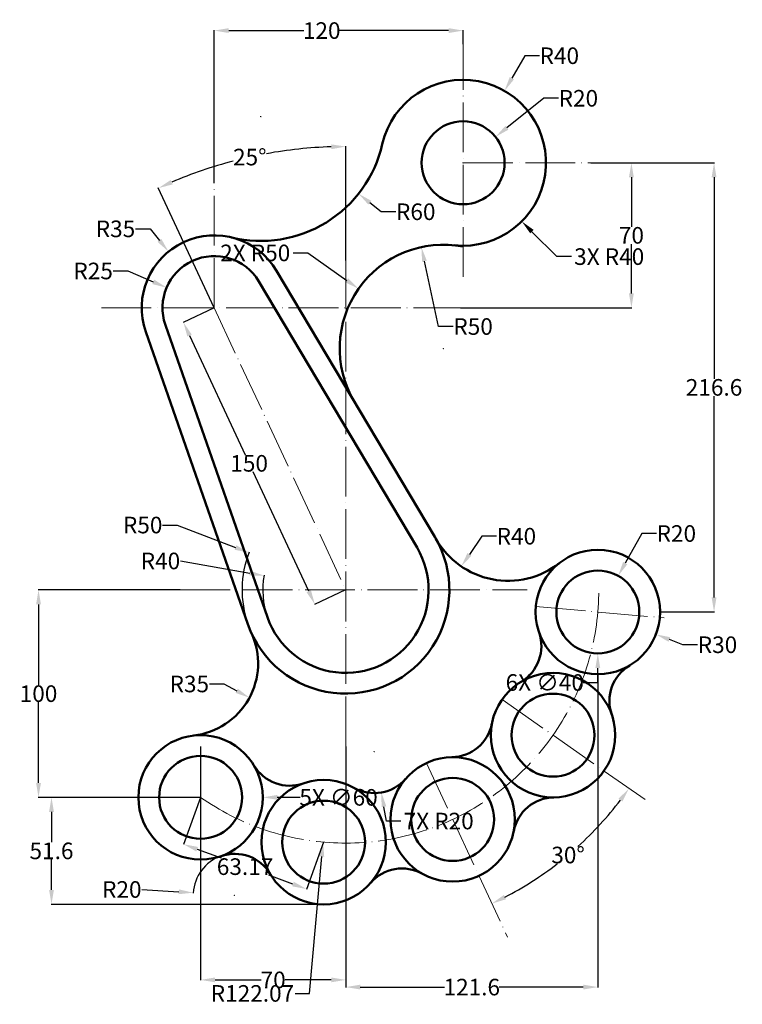
# Model space of a CAD drawing. Units: inches. Extents: x 561 to 910, y 264 to 739.
import ezdxf

# ---------------------------------------------------------------- set-up
doc = ezdxf.new("R2010")
doc.units = ezdxf.units.IN
doc.header["$MEASUREMENT"] = 0
doc.linetypes.add('ACAD_ISO04W100', pattern=[30, 24, -3, 0, -3])
for name, color, linetype, lineweight in [('M-CNTR', 4, 'ACAD_ISO04W100', 18), ('M-DIMS', 2, 'Continuous', 25), ('M-OUTL', 7, 'Continuous', 50)]:
    doc.layers.add(name, color=color, linetype=linetype, lineweight=lineweight)
doc.styles.get("Standard").update_dxf_attribs({"font": 'arial.ttf'})
doc.dimstyles.get("Standard").update_dxf_attribs({"dimtxt": 8, "dimasz": 7, "dimexe": 0.18, "dimexo": 0.0625, "dimgap": 0.09, "dimtad": 0, "dimtih": 1, "dimtoh": 1, "dimdec": 0, "dimzin": 0, "dimdsep": 46, "dimtxsty": 'Standard', "dimcen": 0.09, "dimclrd": 1, "dimclre": 1, "dimadec": 0, "dimazin": 0, "dimtfac": 1, "dimtdec": 0, "dimtofl": 0, "dimtmove": 0, "dimatfit": 3, "dimfxl": 1, "dimtolj": 1, "dimtzin": 0, "dimarcsym": 0})

# ---------------------------------------------------------------- blocks, each defined once
blk = doc.blocks.new('*D1')
at = {"layer": 'Defpoints', "color": 0, "transparency": 16777216}
for p in [(775.26, 733.62), (775.26, 727.02), (655.26, 660.02)]:
    blk.add_point(p, dxfattribs=at)
at = {"layer": 'M-DIMS', "color": 0, "lineweight": -2, "transparency": 16777216}
for p, q in [((655.26, 660.08), (655.26, 733.8)), ((662.26, 733.62), (698.53, 733.62)), ((768.26, 733.62), (715.6, 733.62)), ((775.26, 727.08), (775.26, 733.8))]:
    blk.add_line(p, q, dxfattribs=at)
at = {"layer": 'M-DIMS', "color": 0, "transparency": 16777216}
for points in [[(662.26, 734.79), (662.26, 732.46), (655.26, 733.62)], [(768.26, 734.79), (768.26, 732.46), (775.26, 733.62)]]:
    blk.add_solid(points, dxfattribs=at)
at = {"layer": 'M-DIMS', "color": 0, "transparency": 16777216, "insert": (707.07, 733.62), "char_height": 8, "attachment_point": 5}
blk.add_mtext('\\A1;120', dxfattribs=at)
blk = doc.blocks.new('*D2')
at = {"layer": 'Defpoints', "color": 0, "transparency": 16777216}
for p in [(836.79, 669.91), (856.45, 669.91), (773.89, 599.91)]:
    blk.add_point(p, dxfattribs=at)
at = {"layer": 'M-DIMS', "color": 0, "lineweight": -2, "transparency": 16777216}
for p, q in [((836.85, 669.91), (856.63, 669.91)), ((856.45, 662.91), (856.45, 639.08)), ((856.45, 606.91), (856.45, 630.73)), ((773.95, 599.91), (856.63, 599.91))]:
    blk.add_line(p, q, dxfattribs=at)
at = {"layer": 'M-DIMS', "color": 0, "transparency": 16777216}
for points in [[(855.28, 662.91), (857.61, 662.91), (856.45, 669.91)], [(855.28, 606.91), (857.61, 606.91), (856.45, 599.91)]]:
    blk.add_solid(points, dxfattribs=at)
at = {"layer": 'M-DIMS', "color": 0, "transparency": 16777216, "insert": (856.45, 634.91), "char_height": 8, "attachment_point": 5}
blk.add_mtext('\\A1;70', dxfattribs=at)
blk = doc.blocks.new('*D3')
at = {"layer": 'Defpoints', "color": 0, "transparency": 16777216}
for p in [(677.78, 692.2), (724.83, 654.97)]:
    blk.add_point(p, dxfattribs=at)
at = {"layer": 'M-DIMS', "color": 0, "lineweight": -2, "transparency": 16777216}
for p, q in [((677.69, 692.2), (677.87, 692.2)), ((677.78, 692.11), (677.78, 692.29)), ((735.81, 646.28), (730.32, 650.62)), ((742.81, 646.28), (735.81, 646.28))]:
    blk.add_line(p, q, dxfattribs=at)
at = {"layer": 'M-DIMS', "color": 0, "transparency": 16777216}
blk.add_solid([(731.04, 651.54), (729.59, 649.71), (724.83, 654.97)], dxfattribs=at)
at = {"layer": 'M-DIMS', "color": 0, "transparency": 16777216, "insert": (752.44, 646.28), "char_height": 8, "attachment_point": 5}
blk.add_mtext('\\A1;R60', dxfattribs=at)
blk = doc.blocks.new('*D4')
at = {"layer": 'Defpoints', "color": 0, "transparency": 16777216}
for p in [(755.15, 629.27), (765.75, 580.41)]:
    blk.add_point(p, dxfattribs=at)
at = {"layer": 'M-DIMS', "color": 0, "lineweight": -2, "transparency": 16777216}
for p, q in [((763.47, 590.95), (756.63, 622.43)), ((770.47, 590.95), (763.47, 590.95))]:
    blk.add_line(p, q, dxfattribs=at)
at = {"layer": 'M-DIMS', "color": 0, "transparency": 16777216}
blk.add_solid([(757.77, 622.68), (755.49, 622.19), (755.15, 629.27)], dxfattribs=at)
at = {"layer": 'M-DIMS', "color": 0, "transparency": 16777216, "insert": (780.1, 590.95), "char_height": 8, "attachment_point": 5}
blk.add_mtext('\\A1;R50', dxfattribs=at)
blk = doc.blocks.new('*D5')
at = {"layer": 'Defpoints', "color": 0, "transparency": 16777216}
for p in [(795.26, 704.55), (775.26, 669.91)]:
    blk.add_point(p, dxfattribs=at)
at = {"layer": 'M-DIMS', "color": 0, "lineweight": -2, "transparency": 16777216}
for p, q in [((805.05, 721.5), (798.76, 710.61)), ((812.05, 721.5), (805.05, 721.5)), ((775.17, 669.91), (775.35, 669.91)), ((775.26, 669.82), (775.26, 670))]:
    blk.add_line(p, q, dxfattribs=at)
at = {"layer": 'M-DIMS', "color": 0, "transparency": 16777216}
blk.add_solid([(797.75, 711.2), (799.77, 710.03), (795.26, 704.55)], dxfattribs=at)
at = {"layer": 'M-DIMS', "color": 0, "transparency": 16777216, "insert": (821.68, 721.5), "char_height": 8, "attachment_point": 5}
blk.add_mtext('\\A1;R40', dxfattribs=at)
blk = doc.blocks.new('*D6')
at = {"layer": 'Defpoints', "color": 0, "transparency": 16777216}
for p in [(790.9, 682.38), (775.26, 669.91)]:
    blk.add_point(p, dxfattribs=at)
at = {"layer": 'M-DIMS', "color": 0, "lineweight": -2, "transparency": 16777216}
for p, q in [((814.23, 700.98), (796.37, 686.74)), ((821.23, 700.98), (814.23, 700.98)), ((775.17, 669.91), (775.35, 669.91)), ((775.26, 669.82), (775.26, 670))]:
    blk.add_line(p, q, dxfattribs=at)
at = {"layer": 'M-DIMS', "color": 0, "transparency": 16777216}
blk.add_solid([(795.65, 687.65), (797.1, 685.83), (790.9, 682.38)], dxfattribs=at)
at = {"layer": 'M-DIMS', "color": 0, "transparency": 16777216, "insert": (830.87, 700.98), "char_height": 8, "attachment_point": 5}
blk.add_mtext('\\A1;R20', dxfattribs=at)
blk = doc.blocks.new('*D7')
at = {"layer": 'Defpoints', "color": 0, "transparency": 16777216}
for p in [(687.68, 675.45), (718.66, 622.65), (655.26, 599.91), (718.66, 463.96), (718.66, 388.61)]:
    blk.add_point(p, dxfattribs=at)
at = {"layer": 'M-DIMS', "color": 0, "lineweight": -2, "transparency": 16777216}
for p, q in [((718.66, 622.71), (718.66, 677.89)), ((655.24, 599.96), (628.25, 657.85))]:
    blk.add_line(p, q, dxfattribs=at)
for start, end in [(91.8764, 100.3108), (104.7079, 113.1236)]:
    blk.add_arc((718.66, 463.96), 213.75, start, end, dxfattribs=at)
at = {"layer": 'M-DIMS', "color": 0, "transparency": 16777216}
for points in [[(711.64, 678.76), (711.68, 676.43), (718.66, 677.71)], [(635.19, 659.47), (634.24, 661.6), (628.32, 657.68)]]:
    blk.add_solid(points, dxfattribs=at)
at = {"layer": 'M-DIMS', "color": 0, "transparency": 16777216, "insert": (672.39, 672.64), "char_height": 8, "attachment_point": 5}
blk.add_mtext('\\A1;25°', dxfattribs=at)
blk = doc.blocks.new('*D8')
at = {"layer": 'Defpoints', "color": 0, "transparency": 16777216}
for p in [(633.19, 627.07), (655.26, 599.91)]:
    blk.add_point(p, dxfattribs=at)
at = {"layer": 'M-DIMS', "color": 0, "lineweight": -2, "transparency": 16777216}
for p, q in [((617.29, 638.04), (624.29, 638.04)), ((624.29, 638.04), (628.78, 632.5)), ((655.17, 599.91), (655.35, 599.91)), ((655.26, 599.82), (655.26, 600))]:
    blk.add_line(p, q, dxfattribs=at)
at = {"layer": 'M-DIMS', "color": 0, "transparency": 16777216}
blk.add_solid([(629.69, 633.24), (627.87, 631.77), (633.19, 627.07)], dxfattribs=at)
at = {"layer": 'M-DIMS', "color": 0, "transparency": 16777216, "insert": (607.61, 638.04), "char_height": 8, "attachment_point": 5}
blk.add_mtext('\\A1;R35', dxfattribs=at)
blk = doc.blocks.new('*D9')
at = {"layer": 'Defpoints', "color": 0, "transparency": 16777216}
for p in [(632.27, 609.72), (655.26, 599.91)]:
    blk.add_point(p, dxfattribs=at)
at = {"layer": 'M-DIMS', "color": 0, "lineweight": -2, "transparency": 16777216}
for p, q in [((606.52, 617.73), (613.52, 617.73)), ((613.52, 617.73), (625.83, 612.47)), ((655.17, 599.91), (655.35, 599.91)), ((655.26, 599.82), (655.26, 600))]:
    blk.add_line(p, q, dxfattribs=at)
at = {"layer": 'M-DIMS', "color": 0, "transparency": 16777216}
blk.add_solid([(626.29, 613.54), (625.38, 611.4), (632.27, 609.72)], dxfattribs=at)
at = {"layer": 'M-DIMS', "color": 0, "transparency": 16777216, "insert": (596.84, 617.73), "char_height": 8, "attachment_point": 5}
blk.add_mtext('\\A1;R25', dxfattribs=at)
blk = doc.blocks.new('*D10')
at = {"layer": 'Defpoints', "color": 0, "transparency": 16777216}
for p in [(655.26, 599.91), (718.66, 463.96), (703.77, 457.02)]:
    blk.add_point(p, dxfattribs=at)
at = {"layer": 'M-DIMS', "color": 0, "lineweight": -2, "transparency": 16777216}
for p, q in [((655.21, 599.88), (640.21, 592.89)), ((643.33, 586.62), (670.12, 529.17)), ((700.81, 463.36), (674.02, 520.82)), ((718.6, 463.93), (703.6, 456.94))]:
    blk.add_line(p, q, dxfattribs=at)
at = {"layer": 'M-DIMS', "color": 0, "transparency": 16777216}
for points in [[(644.39, 587.11), (642.27, 586.13), (640.37, 592.96)], [(701.87, 463.85), (699.75, 462.87), (703.77, 457.02)]]:
    blk.add_solid(points, dxfattribs=at)
at = {"layer": 'M-DIMS', "color": 0, "transparency": 16777216, "insert": (672.07, 524.99), "char_height": 8, "attachment_point": 5}
blk.add_mtext('\\A1;150', dxfattribs=at)
blk = doc.blocks.new('*D11')
at = {"layer": 'Defpoints', "color": 0, "transparency": 16777216}
for p in [(671.99, 481.92), (718.66, 463.96)]:
    blk.add_point(p, dxfattribs=at)
at = {"layer": 'M-DIMS', "color": 0, "lineweight": -2, "transparency": 16777216}
for p, q in [((630.36, 495.25), (637.36, 495.25)), ((637.36, 495.25), (665.46, 484.43)), ((718.57, 463.96), (718.75, 463.96)), ((718.66, 463.87), (718.66, 464.05))]:
    blk.add_line(p, q, dxfattribs=at)
blk.add_arc((718.66, 463.96), 50, 158.745, 199.1892, dxfattribs=at)
at = {"layer": 'M-DIMS', "color": 0, "transparency": 16777216}
blk.add_solid([(665.88, 485.52), (665.04, 483.34), (671.99, 481.92)], dxfattribs=at)
at = {"layer": 'M-DIMS', "color": 0, "transparency": 16777216, "insert": (620.73, 495.25), "char_height": 8, "attachment_point": 5}
blk.add_mtext('\\A1;R50', dxfattribs=at)
blk = doc.blocks.new('*D12')
at = {"layer": 'Defpoints', "color": 0, "transparency": 16777216}
for p in [(679.26, 470.87), (718.66, 463.96)]:
    blk.add_point(p, dxfattribs=at)
at = {"layer": 'M-DIMS', "color": 0, "lineweight": -2, "transparency": 16777216}
for p, q in [((638.94, 477.93), (672.36, 472.07)), ((718.57, 463.96), (718.75, 463.96)), ((718.66, 463.87), (718.66, 464.05))]:
    blk.add_line(p, q, dxfattribs=at)
blk.add_arc((718.66, 463.96), 40, 169.8016, 199.1713, dxfattribs=at)
at = {"layer": 'M-DIMS', "color": 0, "transparency": 16777216}
blk.add_solid([(672.56, 473.22), (672.16, 470.93), (679.26, 470.87)], dxfattribs=at)
at = {"layer": 'M-DIMS', "color": 0, "transparency": 16777216, "insert": (629.3, 477.93), "char_height": 8, "attachment_point": 5}
blk.add_mtext('\\A1;R40', dxfattribs=at)
blk = doc.blocks.new('*D13')
at = {"layer": 'Defpoints', "color": 0, "transparency": 16777216}
for p in [(796.96, 508.33), (774.38, 475.31)]:
    blk.add_point(p, dxfattribs=at)
at = {"layer": 'M-DIMS', "color": 0, "lineweight": -2, "transparency": 16777216}
for p, q in [((784.34, 489.86), (778.33, 481.09)), ((791.34, 489.86), (784.34, 489.86))]:
    blk.add_line(p, q, dxfattribs=at)
at = {"layer": 'M-DIMS', "color": 0, "transparency": 16777216}
blk.add_solid([(777.37, 481.75), (779.3, 480.43), (774.38, 475.31)], dxfattribs=at)
at = {"layer": 'M-DIMS', "color": 0, "transparency": 16777216, "insert": (800.97, 489.86), "char_height": 8, "attachment_point": 5}
blk.add_mtext('\\A1;R40', dxfattribs=at)
blk = doc.blocks.new('*D14')
at = {"layer": 'Defpoints', "color": 0, "transparency": 16777216}
for p in [(641.38, 428.55), (672.23, 412.02)]:
    blk.add_point(p, dxfattribs=at)
at = {"layer": 'M-DIMS', "color": 0, "lineweight": -2, "transparency": 16777216}
for p, q in [((652.89, 418.63), (659.89, 418.63)), ((659.89, 418.63), (666.06, 415.33))]:
    blk.add_line(p, q, dxfattribs=at)
at = {"layer": 'M-DIMS', "color": 0, "transparency": 16777216}
blk.add_solid([(666.61, 416.36), (665.51, 414.3), (672.23, 412.02)], dxfattribs=at)
at = {"layer": 'M-DIMS', "color": 0, "transparency": 16777216, "insert": (643.22, 418.63), "char_height": 8, "attachment_point": 5}
blk.add_mtext('\\A1;R35', dxfattribs=at)
blk = doc.blocks.new('*D15')
at = {"layer": 'Defpoints', "color": 0, "transparency": 16777216}
for p in [(638.93, 463.96), (570.49, 363.96), (648.66, 363.96)]:
    blk.add_point(p, dxfattribs=at)
at = {"layer": 'M-DIMS', "color": 0, "lineweight": -2, "transparency": 16777216}
for p, q in [((638.87, 463.96), (570.31, 463.96)), ((570.49, 456.96), (570.49, 418.14)), ((570.49, 370.96), (570.49, 409.79)), ((648.59, 363.96), (570.31, 363.96))]:
    blk.add_line(p, q, dxfattribs=at)
at = {"layer": 'M-DIMS', "color": 0, "transparency": 16777216}
for points in [[(569.32, 456.96), (571.66, 456.96), (570.49, 463.96)], [(569.32, 370.96), (571.66, 370.96), (570.49, 363.96)]]:
    blk.add_solid(points, dxfattribs=at)
at = {"layer": 'M-DIMS', "color": 0, "transparency": 16777216, "insert": (570.49, 413.96), "char_height": 8, "attachment_point": 5}
blk.add_mtext('\\A1;100', dxfattribs=at)
blk = doc.blocks.new('*D16')
at = {"layer": 'Defpoints', "color": 0, "transparency": 16777216}
for p in [(850.04, 470.76), (840.26, 453.32)]:
    blk.add_point(p, dxfattribs=at)
at = {"layer": 'M-DIMS', "color": 0, "lineweight": -2, "transparency": 16777216}
for p, q in [((861.49, 491.16), (853.47, 476.87)), ((868.49, 491.16), (861.49, 491.16)), ((840.17, 453.32), (840.35, 453.32)), ((840.26, 453.23), (840.26, 453.41))]:
    blk.add_line(p, q, dxfattribs=at)
at = {"layer": 'M-DIMS', "color": 0, "transparency": 16777216}
blk.add_solid([(852.45, 477.44), (854.49, 476.3), (850.04, 470.76)], dxfattribs=at)
at = {"layer": 'M-DIMS', "color": 0, "transparency": 16777216, "insert": (878.12, 491.16), "char_height": 8, "attachment_point": 5}
blk.add_mtext('\\A1;R20', dxfattribs=at)
blk = doc.blocks.new('*D17')
at = {"layer": 'Defpoints', "color": 0, "transparency": 16777216}
for p in [(840.26, 453.32), (868.26, 442.56)]:
    blk.add_point(p, dxfattribs=at)
at = {"layer": 'M-DIMS', "color": 0, "lineweight": -2, "transparency": 16777216}
for p, q in [((840.17, 453.32), (840.35, 453.32)), ((840.26, 453.23), (840.26, 453.41)), ((881.33, 437.54), (874.8, 440.05)), ((888.33, 437.54), (881.33, 437.54))]:
    blk.add_line(p, q, dxfattribs=at)
at = {"layer": 'M-DIMS', "color": 0, "transparency": 16777216}
blk.add_solid([(875.21, 441.14), (874.38, 438.96), (868.26, 442.56)], dxfattribs=at)
at = {"layer": 'M-DIMS', "color": 0, "transparency": 16777216, "insert": (897.97, 437.54), "char_height": 8, "attachment_point": 5}
blk.add_mtext('\\A1;R30', dxfattribs=at)
blk = doc.blocks.new('*D18')
at = {"layer": 'Defpoints', "color": 0, "transparency": 16777216}
for p in [(794.07, 411.15), (757.57, 380.52), (864.91, 361.55), (814.35, 327.3), (796.73, 296.54)]:
    blk.add_point(p, dxfattribs=at)
at = {"layer": 'M-DIMS', "color": 0, "lineweight": -2, "transparency": 16777216}
for start, end in [(312.1829, 322.5957), (297.4043, 307.7131)]:
    blk.add_arc((718.66, 463.96), 166.83, start, end, dxfattribs=at)
at = {"layer": 'M-DIMS', "color": 0, "transparency": 16777216}
for points in [[(850.24, 363.31), (852.12, 361.94), (855.31, 368.27)], [(795.96, 314.81), (794.93, 316.9), (789.16, 312.76)]]:
    blk.add_solid(points, dxfattribs=at)
at = {"layer": 'M-DIMS', "color": 0, "transparency": 16777216, "insert": (825.89, 336.16), "char_height": 8, "attachment_point": 5}
blk.add_mtext('\\A1;30°', dxfattribs=at)
blk = doc.blocks.new('*D19')
at = {"layer": 'Defpoints', "color": 0, "transparency": 16777216}
for p in [(648.66, 388.61), (718.66, 388.61), (648.66, 275.95)]:
    blk.add_point(p, dxfattribs=at)
at = {"layer": 'M-DIMS', "color": 0, "lineweight": -2, "transparency": 16777216}
for p, q in [((648.66, 388.55), (648.66, 275.77)), ((718.66, 388.55), (718.66, 275.77)), ((655.66, 275.95), (677.88, 275.95)), ((711.66, 275.95), (689.43, 275.95))]:
    blk.add_line(p, q, dxfattribs=at)
at = {"layer": 'M-DIMS', "color": 0, "transparency": 16777216}
for points in [[(655.66, 277.12), (655.66, 274.79), (648.66, 275.95)], [(711.66, 277.12), (711.66, 274.79), (718.66, 275.95)]]:
    blk.add_solid(points, dxfattribs=at)
at = {"layer": 'M-DIMS', "color": 0, "transparency": 16777216, "insert": (683.66, 275.95), "char_height": 8, "attachment_point": 5}
blk.add_mtext('\\A1;70', dxfattribs=at)
blk = doc.blocks.new('*D20')
at = {"layer": 'Defpoints', "color": 0, "transparency": 16777216}
for p in [(645.12, 317.99), (665.08, 316.74)]:
    blk.add_point(p, dxfattribs=at)
at = {"layer": 'M-DIMS', "color": 0, "lineweight": -2, "transparency": 16777216}
for p, q in [((620.29, 319.55), (638.14, 318.43)), ((664.99, 316.74), (665.17, 316.74)), ((665.08, 316.65), (665.08, 316.83))]:
    blk.add_line(p, q, dxfattribs=at)
blk.add_arc((665.08, 316.74), 20, 109.3582, 176.9159, dxfattribs=at)
at = {"layer": 'M-DIMS', "color": 0, "transparency": 16777216}
blk.add_solid([(638.21, 319.6), (638.06, 317.27), (645.12, 317.99)], dxfattribs=at)
at = {"layer": 'M-DIMS', "color": 0, "transparency": 16777216, "insert": (610.66, 319.55), "char_height": 8, "attachment_point": 5}
blk.add_mtext('\\A1;R20', dxfattribs=at)
blk = doc.blocks.new('MOUNT-NODE-OD60-ID40')
for radius in [30, 20]:
    blk.add_circle((30, 30), radius)
blk = doc.blocks.new('*D22')
at = {"layer": 'Defpoints', "color": 0, "transparency": 16777216}
for p in [(840.26, 423.32), (718.66, 388.61), (840.26, 272.49)]:
    blk.add_point(p, dxfattribs=at)
at = {"layer": 'M-DIMS', "color": 1, "lineweight": -2, "transparency": 16777216}
for p, q in [((840.26, 423.26), (840.26, 272.31)), ((718.66, 388.55), (718.66, 272.31)), ((725.66, 272.49), (766.25, 272.49)), ((833.26, 272.49), (792.67, 272.49))]:
    blk.add_line(p, q, dxfattribs=at)
at = {"layer": 'M-DIMS', "color": 1, "transparency": 16777216}
for points in [[(725.66, 273.66), (725.66, 271.33), (718.66, 272.49)], [(833.26, 273.66), (833.26, 271.33), (840.26, 272.49)]]:
    blk.add_solid(points, dxfattribs=at)
at = {"layer": 'M-DIMS', "color": 0, "transparency": 16777216, "insert": (779.46, 272.49), "char_height": 8, "attachment_point": 5}
blk.add_mtext('\\A1;121.6', dxfattribs=at)
blk = doc.blocks.new('*D23')
at = {"layer": 'Defpoints', "color": 0, "transparency": 16777216}
for p in [(618.66, 363.96), (576.75, 312.36), (708.02, 312.36)]:
    blk.add_point(p, dxfattribs=at)
at = {"layer": 'M-DIMS', "color": 1, "lineweight": -2, "transparency": 16777216}
for p, q in [((618.59, 363.96), (576.57, 363.96)), ((576.75, 356.96), (576.75, 342.34)), ((576.75, 319.36), (576.75, 333.99)), ((707.96, 312.36), (576.57, 312.36))]:
    blk.add_line(p, q, dxfattribs=at)
at = {"layer": 'M-DIMS', "color": 1, "transparency": 16777216}
for points in [[(575.58, 356.96), (577.91, 356.96), (576.75, 363.96)], [(575.58, 319.36), (577.91, 319.36), (576.75, 312.36)]]:
    blk.add_solid(points, dxfattribs=at)
at = {"layer": 'M-DIMS', "color": 0, "transparency": 16777216, "insert": (576.75, 338.16), "char_height": 8, "attachment_point": 5}
blk.add_mtext('\\A1;51.6', dxfattribs=at)
blk = doc.blocks.new('*D24')
at = {"layer": 'Defpoints', "color": 0, "transparency": 16777216}
for p in [(836.79, 669.91), (870.26, 453.32), (896.31, 453.32)]:
    blk.add_point(p, dxfattribs=at)
at = {"layer": 'M-DIMS', "color": 1, "lineweight": -2, "transparency": 16777216}
for p, q in [((836.85, 669.91), (896.49, 669.91)), ((896.31, 662.91), (896.31, 565.79)), ((896.31, 460.32), (896.31, 557.44)), ((870.32, 453.32), (896.49, 453.32))]:
    blk.add_line(p, q, dxfattribs=at)
at = {"layer": 'M-DIMS', "color": 1, "transparency": 16777216}
for points in [[(895.14, 662.91), (897.48, 662.91), (896.31, 669.91)], [(895.14, 460.32), (897.48, 460.32), (896.31, 453.32)]]:
    blk.add_solid(points, dxfattribs=at)
at = {"layer": 'M-DIMS', "color": 0, "transparency": 16777216, "insert": (896.31, 561.61), "char_height": 8, "attachment_point": 5}
blk.add_mtext('\\A1;216.6', dxfattribs=at)
blk = doc.blocks.new('*D25')
at = {"layer": 'Defpoints', "color": 0, "transparency": 16777216}
for p in [(648.66, 363.96), (708.02, 342.36), (640.43, 341.36)]:
    blk.add_point(p, dxfattribs=at)
at = {"layer": 'M-DIMS', "color": 1, "lineweight": -2, "transparency": 16777216}
for p, q in [((648.64, 363.9), (640.37, 341.19)), ((708, 342.3), (699.73, 319.59)), ((647.01, 338.97), (658.63, 334.74)), ((693.22, 322.15), (681.59, 326.38))]:
    blk.add_line(p, q, dxfattribs=at)
at = {"layer": 'M-DIMS', "color": 1, "transparency": 16777216}
for points in [[(647.41, 340.06), (646.61, 337.87), (640.43, 341.36)], [(693.62, 323.25), (692.82, 321.06), (699.79, 319.76)]]:
    blk.add_solid(points, dxfattribs=at)
at = {"layer": 'M-DIMS', "color": 0, "transparency": 16777216, "insert": (670.11, 330.56), "char_height": 8, "attachment_point": 5}
blk.add_mtext('\\A1;63.17', dxfattribs=at)
blk = doc.blocks.new('*D26')
at = {"layer": 'Defpoints', "color": 0, "transparency": 16777216}
for p in [(718.66, 463.96), (707.75, 342.38)]:
    blk.add_point(p, dxfattribs=at)
at = {"layer": 'M-DIMS', "color": 1, "lineweight": -2, "transparency": 16777216}
for p, q in [((718.57, 463.96), (718.75, 463.96)), ((718.66, 463.87), (718.66, 464.05)), ((701.21, 269.44), (707.12, 335.41)), ((694.21, 269.44), (701.21, 269.44))]:
    blk.add_line(p, q, dxfattribs=at)
at = {"layer": 'M-DIMS', "color": 1, "transparency": 16777216}
blk.add_solid([(705.96, 335.52), (708.29, 335.31), (707.75, 342.38)], dxfattribs=at)
at = {"layer": 'M-DIMS', "color": 0, "transparency": 16777216, "insert": (673.68, 269.44), "char_height": 8, "attachment_point": 5}
blk.add_mtext('\\A1;R122.07', dxfattribs=at)
blk = doc.blocks.new('*D27')
at = {"layer": 'Defpoints', "color": 0, "transparency": 16777216}
for p in [(724.85, 609.17), (765.75, 580.41)]:
    blk.add_point(p, dxfattribs=at)
at = {"layer": 'M-DIMS', "color": 1, "lineweight": -2, "transparency": 16777216}
for p, q in [((693.31, 626.43), (700.31, 626.43)), ((700.31, 626.43), (719.13, 613.2)), ((765.66, 580.41), (765.84, 580.41)), ((765.75, 580.32), (765.75, 580.5))]:
    blk.add_line(p, q, dxfattribs=at)
at = {"layer": 'M-DIMS', "color": 1, "transparency": 16777216}
blk.add_solid([(719.8, 614.15), (718.45, 612.24), (724.85, 609.17)], dxfattribs=at)
at = {"layer": 'M-DIMS', "color": 0, "transparency": 16777216, "insert": (675.01, 626.43), "char_height": 8, "attachment_point": 5}
blk.add_mtext('\\A1;2X R50', dxfattribs=at)
blk = doc.blocks.new('*D28')
at = {"layer": 'Defpoints', "color": 0, "transparency": 16777216}
for p in [(775.26, 669.91), (803.55, 641.62)]:
    blk.add_point(p, dxfattribs=at)
at = {"layer": 'M-DIMS', "color": 1, "lineweight": -2, "transparency": 16777216}
for p, q in [((775.17, 669.91), (775.35, 669.91)), ((775.26, 669.82), (775.26, 670)), ((820.52, 624.65), (808.5, 636.67)), ((827.52, 624.65), (820.52, 624.65))]:
    blk.add_line(p, q, dxfattribs=at)
at = {"layer": 'M-DIMS', "color": 1, "transparency": 16777216}
blk.add_solid([(809.32, 637.5), (807.67, 635.85), (803.55, 641.62)], dxfattribs=at)
at = {"layer": 'M-DIMS', "color": 0, "transparency": 16777216, "insert": (845.74, 624.65), "char_height": 8, "attachment_point": 5}
blk.add_mtext('\\A1;3X R40', dxfattribs=at)
blk = doc.blocks.new('*D29')
at = {"layer": 'Defpoints', "color": 0, "transparency": 16777216}
for p in [(618.66, 363.96), (678.66, 363.96)]:
    blk.add_point(p, dxfattribs=at)
at = {"layer": 'M-DIMS', "color": 1, "lineweight": -2, "transparency": 16777216}
for p, q in [((648.57, 363.96), (648.75, 363.96)), ((648.66, 363.87), (648.66, 364.05)), ((696.66, 363.96), (685.66, 363.96))]:
    blk.add_line(p, q, dxfattribs=at)
at = {"layer": 'M-DIMS', "color": 1, "transparency": 16777216}
blk.add_solid([(685.66, 365.13), (685.66, 362.79), (678.66, 363.96)], dxfattribs=at)
at = {"layer": 'M-DIMS', "color": 0, "transparency": 16777216, "insert": (715.2, 363.96), "char_height": 8, "attachment_point": 5}
blk.add_mtext('\\A1;5X ∅60', dxfattribs=at)
blk = doc.blocks.new('*D30')
at = {"layer": 'Defpoints', "color": 0, "transparency": 16777216}
for p in [(840.27, 473.32), (840.25, 433.32)]:
    blk.add_point(p, dxfattribs=at)
at = {"layer": 'M-DIMS', "color": 1, "lineweight": -2, "transparency": 16777216}
for p, q in [((840.17, 453.32), (840.35, 453.32)), ((840.26, 453.23), (840.26, 453.41)), ((840.24, 419.32), (840.25, 426.32)), ((833.24, 419.32), (840.24, 419.32))]:
    blk.add_line(p, q, dxfattribs=at)
at = {"layer": 'M-DIMS', "color": 1, "transparency": 16777216}
blk.add_solid([(839.08, 426.32), (841.41, 426.32), (840.25, 433.32)], dxfattribs=at)
at = {"layer": 'M-DIMS', "color": 0, "transparency": 16777216, "insert": (814.68, 419.32), "char_height": 8, "attachment_point": 5}
blk.add_mtext('\\A1;6X ∅40', dxfattribs=at)
blk = doc.blocks.new('*D31')
at = {"layer": 'Defpoints', "color": 0, "transparency": 16777216}
for p in [(732.4, 386.01), (735.87, 366.32)]:
    blk.add_point(p, dxfattribs=at)
at = {"layer": 'M-DIMS', "color": 1, "lineweight": -2, "transparency": 16777216}
for p, q in [((732.31, 386.01), (732.49, 386.01)), ((732.4, 385.92), (732.4, 386.1)), ((738.31, 352.53), (737.09, 359.42)), ((745.31, 352.53), (738.31, 352.53))]:
    blk.add_line(p, q, dxfattribs=at)
at = {"layer": 'M-DIMS', "color": 1, "transparency": 16777216}
blk.add_solid([(738.24, 359.62), (735.94, 359.22), (735.87, 366.32)], dxfattribs=at)
at = {"layer": 'M-DIMS', "color": 0, "transparency": 16777216, "insert": (763.5, 352.53), "char_height": 8, "attachment_point": 5}
blk.add_mtext('\\A1;7X R20', dxfattribs=at)

msp = doc.modelspace()

# ---------------------------------------------------------------- linework, layer by layer
at = {"layer": 'M-CNTR'}
for p, q in [((775.265, 614.824), (775.265, 727.022)), ((775.265, 669.907), (836.786, 669.907)), ((655.265, 599.907), (655.265, 660.019)), ((718.657, 388.612), (718.657, 622.648)), ((600.796, 599.907), (773.886, 599.907)), ((655.265, 599.907), (718.657, 463.961)), ((638.929, 463.961), (806.223, 463.961)), ((810.373, 455.937), (872.261, 450.523)), ((794.073, 411.155), (864.91, 361.554)), ((757.566, 380.521), (796.726, 296.542))]:
    msp.add_line(p, q, dxfattribs=at)
msp.add_arc((718.657, 463.961), 122.066, 235.00798, 0, dxfattribs=at)
at = {"layer": 'M-OUTL'}
for p, q in [((685.347, 617.797), (761.632, 489.518)), ((676.752, 612.686), (753.037, 484.406)), ((631.664, 591.661), (680.896, 450.766)), ((622.224, 588.362), (671.456, 447.468))]:
    msp.add_line(p, q, dxfattribs=at)
msp.add_circle((775.265, 669.907), 20, dxfattribs=at)
for centre, radius, start, end in [((775.265, 669.907), 40, 263.9333, 167.11879), ((677.781, 692.2), 60, 256.28948, 347.11879), ((655.265, 599.907), 35, 30.73917, 199.26083), ((765.753, 580.411), 50, 79.03349, 210.73917), ((655.265, 599.907), 25, 30.73917, 199.26083), ((718.657, 463.961), 50, 199.26083, 30.73917), ((718.657, 463.961), 40, 199.26083, 30.73917), ((796.962, 508.327), 40, 209.53468, 308.2076), ((641.383, 428.553), 35, 276.4252, 24.6181), ((793.036, 436.89), 20, 300.81268, 19.18732), ((865.87, 410.38), 20, 120.81268, 199.18732), ((769.535, 403.327), 20, 270.81267, 349.18732), ((691.592, 389.585), 20, 210.82881, 289.17917), ((732.402, 386.012), 20, 240.81268, 319.18732), ((819.357, 343.952), 20, 90.81267, 169.18732), ((665.083, 316.736), 20, 30.82881, 109.17917), ((745.861, 309.681), 20, 60.81268, 139.18732)]:
    msp.add_arc(centre, radius, start, end, dxfattribs=at)

# ---------------------------------------------------------------- block references
for p, rotation in [((867.53, 420.822), 84.99999835422717), ((826.015, 352.165), 55.00000023408051), ((755.734, 313.464), 24.99999867833716), ((675.518, 315.089), 355.0000025459568)]:
    msp.add_blockref('MOUNT-NODE-OD60-ID40', p, dxfattribs=dict(at, rotation=rotation))
msp.add_blockref('MOUNT-NODE-OD60-ID40', (618.657, 333.961), dxfattribs=at)

# ---------------------------------------------------------------- dimensions: what is measured, and where the dimension line sits
at = {"layer": 'M-DIMS'}
dim = msp.add_linear_dim(base=(775.265, 733.622), p1=(655.265, 660.019), p2=(775.265, 727.022), dimstyle='Standard', override={"dimclrd": 0, "dimclre": 0, "dimclrt": 0}, dxfattribs=at)
dim.commit()
dim.dimension.update_dxf_attribs({"geometry": '*D1', "text_midpoint": (707.066, 733.622), "dimtype": 160})
for center, mpoint, override, picture, middle in [((775.265, 669.907), (795.263, 704.55), {"dimclrd": 0, "dimclre": 0, "dimclrt": 0}, '*D5', (821.682, 721.5)), ((775.265, 669.907), (790.902, 682.376), {"dimclrd": 0, "dimclre": 0, "dimclrt": 0}, '*D6', (830.869, 700.982)), ((655.265, 599.907), (633.194, 627.072), {"dimclrd": 0, "dimclre": 0, "dimclrt": 0}, '*D8', (607.609, 638.035)), ((765.753, 580.411), (755.15, 629.274), {"dimclrd": 0, "dimclre": 0, "dimclrt": 0}, '*D4', (780.101, 590.946)), ((655.265, 599.907), (632.272, 609.722), {"dimclrd": 0, "dimclre": 0, "dimclrt": 0}, '*D9', (596.839, 617.728)), ((796.962, 508.327), (774.383, 475.309), {"dimclrd": 0, "dimclre": 0, "dimclrt": 0}, '*D13', (800.969, 489.862)), ((718.657, 463.961), (671.994, 481.919), {"dimclrd": 0, "dimclre": 0, "dimclrt": 0}, '*D11', (620.727, 495.247)), ((840.258, 453.322), (850.045, 470.765), {"dimclrd": 0, "dimclre": 0, "dimclrt": 0}, '*D16', (878.121, 491.157)), ((718.657, 463.961), (679.258, 470.866), {"dimclrd": 0, "dimclre": 0, "dimclrt": 0}, '*D12', (638.937, 477.933)), ((718.657, 463.961), (707.75, 342.384), {"dimdec": 2, "dimlfac": 1, "dimrnd": 0, "dimzin": 0, "dimdsep": 46, "dimlunit": 2}, '*D26', (673.682, 269.438)), ((641.383, 428.553), (672.233, 412.022), {"dimclrd": 0, "dimclre": 0, "dimclrt": 0}, '*D14', (643.215, 418.634)), ((665.083, 316.736), (645.123, 317.992), {"dimclrd": 0, "dimclre": 0, "dimclrt": 0}, '*D20', (620.291, 319.554))]:
    dim = msp.add_radius_dim(center=center, mpoint=mpoint, dimstyle='Standard', override=override, dxfattribs=at)
    dim.commit()
    dim.dimension.update_dxf_attribs({"geometry": picture, "text_midpoint": middle, "dimtype": 164})
for center, mpoint, picture, middle in [((677.781, 692.2), (724.83, 654.965), '*D3', (752.442, 646.277)), ((840.258, 453.322), (868.262, 442.562), '*D17', (897.965, 437.541))]:
    dim = msp.add_radius_dim(center=center, mpoint=mpoint, dimstyle='Standard', override={"dimclrd": 0, "dimclre": 0, "dimclrt": 0}, dxfattribs=at)
    dim.commit()
    dim.dimension.update_dxf_attribs({"geometry": picture, "text_midpoint": middle})
for base, line1, line2, picture, middle in [((687.678, 675.453), ((718.657, 388.612), (718.657, 622.648)), ((655.265, 599.907), (718.657, 463.961)), '*D7', (672.394, 672.644)), ((814.346, 327.304), ((794.073, 411.155), (864.91, 361.554)), ((757.566, 380.521), (796.726, 296.542)), '*D18', (825.892, 336.164))]:
    dim = msp.add_angular_dim_2l(base=base, line1=line1, line2=line2, dimstyle='Standard', override={"dimclrd": 0, "dimclre": 0, "dimclrt": 0}, dxfattribs=at)
    dim.commit()
    dim.dimension.update_dxf_attribs({"geometry": picture, "text_midpoint": middle})
for base, p1, p2, angle, override, picture, middle in [((856.447, 669.907), (773.886, 599.907), (836.786, 669.907), 90, {"dimclrd": 0, "dimclre": 0, "dimclrt": 0}, '*D2', (856.447, 634.907)), ((896.311, 453.322), (836.786, 669.907), (870.258, 453.322), 90, {"dimdec": 1, "dimlfac": 1, "dimrnd": 0, "dimzin": 0, "dimdsep": 46, "dimlunit": 2}, '*D24', (896.311, 561.615)), ((570.491, 363.961), (638.929, 463.961), (648.657, 363.961), 90, {"dimclrd": 0, "dimclre": 0, "dimclrt": 0}, '*D15', (570.491, 413.961)), ((576.746, 312.36), (618.657, 363.961), (708.019, 312.36), 90, {"dimdec": 1, "dimlfac": 1, "dimrnd": 0, "dimzin": 0, "dimdsep": 46, "dimlunit": 2}, '*D23', (576.746, 338.161)), ((640.433, 341.361), (708.019, 342.36), (648.657, 363.961), 160.00399, {"dimdec": 2, "dimlfac": 1, "dimrnd": 0, "dimzin": 0, "dimdsep": 46, "dimlunit": 2}, '*D25', (670.114, 330.56))]:
    dim = msp.add_linear_dim(base=base, p1=p1, p2=p2, angle=angle, dimstyle='Standard', override=override, dxfattribs=at)
    dim.commit()
    dim.dimension.update_dxf_attribs({"geometry": picture, "text_midpoint": middle})
for center, mpoint, text, picture, middle in [((775.265, 669.907), (803.548, 641.622), '3X <>', '*D28', (845.744, 624.651)), ((765.753, 580.411), (724.852, 609.171), '2X <>', '*D27', (675.014, 626.427))]:
    dim = msp.add_radius_dim(center=center, mpoint=mpoint, text=text, dimstyle='Standard', override={"dimdec": 0, "dimlfac": 1, "dimrnd": 0, "dimzin": 0, "dimdsep": 46, "dimlunit": 2}, dxfattribs=at)
    dim.commit()
    dim.dimension.update_dxf_attribs({"geometry": picture, "text_midpoint": middle, "dimtype": 164})
dim = msp.add_aligned_dim(p1=(655.265, 599.907), p2=(718.657, 463.961), distance=-16.43, dimstyle='Standard', override={"dimclrd": 0, "dimclre": 0, "dimclrt": 0}, dxfattribs=at)
dim.commit()
dim.dimension.update_dxf_attribs({"geometry": '*D10', "text_midpoint": (672.07, 524.99)})
for p1, p2, text, picture, middle in [((840.267, 473.322), (840.25, 433.322), '6X <>', '*D30', (814.682, 419.322)), ((618.657, 363.961), (678.657, 363.961), '5X <>', '*D29', (696.657, 363.961))]:
    dim = msp.add_diameter_dim_2p(p1=p1, p2=p2, text=text, dimstyle='Standard', override={"dimdec": 0, "dimlfac": 1, "dimrnd": 0, "dimzin": 0, "dimdsep": 46, "dimlunit": 2}, dxfattribs=at)
    dim.commit()
    dim.dimension.update_dxf_attribs({"geometry": picture, "text_midpoint": middle, "dimtype": 163})
for base, p2, override, picture, middle in [((840.258, 272.492), (840.258, 423.322), {"dimdec": 1, "dimlfac": 1, "dimrnd": 0, "dimzin": 0, "dimdsep": 46, "dimlunit": 2}, '*D22', (779.458, 272.492)), ((648.657, 275.954), (648.657, 388.612), {"dimclrd": 0, "dimclre": 0, "dimclrt": 0}, '*D19', (683.657, 275.954))]:
    dim = msp.add_linear_dim(base=base, p1=(718.657, 388.612), p2=p2, dimstyle='Standard', override=override, dxfattribs=at)
    dim.commit()
    dim.dimension.update_dxf_attribs({"geometry": picture, "text_midpoint": middle})
dim = msp.add_radius_dim(center=(732.402, 386.012), mpoint=(735.875, 366.315), text='7X <>', dimstyle='Standard', override={"dimdec": 0, "dimlfac": 1, "dimrnd": 0, "dimzin": 0, "dimdsep": 46, "dimlunit": 2}, dxfattribs=at)
dim.commit()
dim.dimension.update_dxf_attribs({"geometry": '*D31', "text_midpoint": (763.502, 352.528)})

doc.saveas('drawing.dxf')
